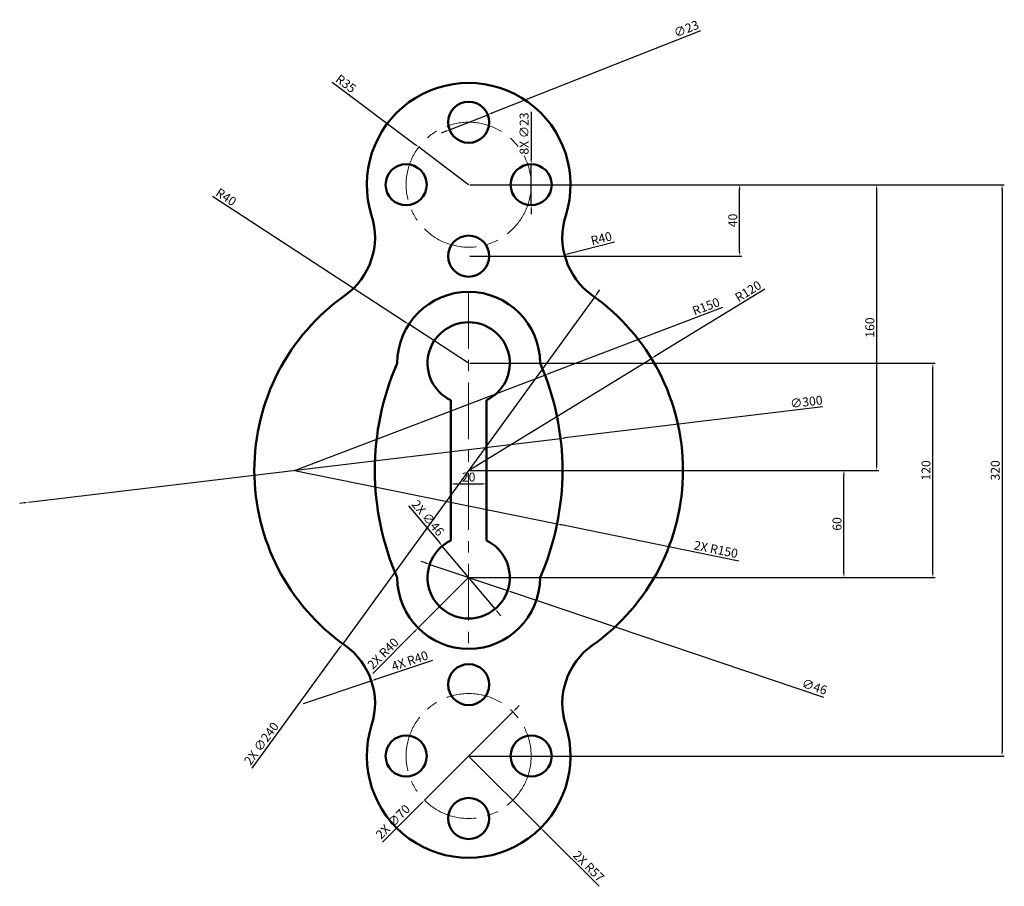
# Model space of a CAD drawing. Units: millimetres. Extents: x 3115 to 3666, y 1639 to 2124.
import ezdxf

# ---------------------------------------------------------------- set-up
doc = ezdxf.new("R2010")
doc.units = ezdxf.units.MM
doc.linetypes.add('CENTER', pattern=[50.8, 31.75, -6.35, 6.35, -6.35])
for name, color, linetype, lineweight in [('M-CNTR', 4, 'CENTER', 18), ('M-DIMS', 2, 'Continuous', 25), ('M-OUTL', 7, 'Continuous', 50)]:
    doc.layers.add(name, color=color, linetype=linetype, lineweight=lineweight)
doc.styles.get("Standard").update_dxf_attribs({"font": 'arial.ttf'})
doc.dimstyles.new('ISO-25', dxfattribs={"dimtxt": 5, "dimasz": 2.5, "dimexe": 1.25, "dimexo": 0.625, "dimtad": 1, "dimtxsty": 'Standard', "dimcen": 2.5, "dimadec": 0, "dimazin": 0, "dimtfac": 1, "dimtmove": 0, "dimatfit": 3, "dimfxl": 1, "dimarcsym": 0})

# ---------------------------------------------------------------- blocks, each defined once
blk = doc.blocks.new('*D1')
at = {"layer": 'Defpoints', "color": 0, "transparency": 16777216}
for p in [(3366.01, 1931.75), (3625.89, 1931.75), (3366.01, 1811.75)]:
    blk.add_point(p, dxfattribs=at)
at = {"layer": 'M-DIMS', "color": 0, "lineweight": -2, "transparency": 16777216}
for p, q in [((3366.63, 1931.75), (3627.14, 1931.75)), ((3625.89, 1814.25), (3625.89, 1929.25)), ((3366.63, 1811.75), (3627.14, 1811.75))]:
    blk.add_line(p, q, dxfattribs=at)
at = {"layer": 'M-DIMS', "color": 0, "transparency": 16777216}
for points in [[(3625.47, 1929.25), (3626.3, 1929.25), (3625.89, 1931.75)], [(3625.47, 1814.25), (3626.3, 1814.25), (3625.89, 1811.75)]]:
    blk.add_solid(points, dxfattribs=at)
at = {"layer": 'M-DIMS', "color": 0, "transparency": 16777216, "insert": (3622.71, 1871.75), "char_height": 5, "attachment_point": 5, "rotation": 90}
blk.add_mtext('120', dxfattribs=at)
blk = doc.blocks.new('*D2')
at = {"layer": 'Defpoints', "color": 0, "transparency": 16777216}
for p in [(3366.01, 1871.75), (3576.08, 1871.75), (3366.01, 1811.75)]:
    blk.add_point(p, dxfattribs=at)
at = {"layer": 'M-DIMS', "color": 0, "lineweight": -2, "transparency": 16777216}
for p, q in [((3366.63, 1871.75), (3577.33, 1871.75)), ((3576.08, 1814.25), (3576.08, 1869.25)), ((3366.63, 1811.75), (3577.33, 1811.75))]:
    blk.add_line(p, q, dxfattribs=at)
at = {"layer": 'M-DIMS', "color": 0, "transparency": 16777216}
for points in [[(3575.66, 1869.25), (3576.5, 1869.25), (3576.08, 1871.75)], [(3575.66, 1814.25), (3576.5, 1814.25), (3576.08, 1811.75)]]:
    blk.add_solid(points, dxfattribs=at)
at = {"layer": 'M-DIMS', "color": 0, "transparency": 16777216, "insert": (3572.9, 1841.75), "char_height": 5, "attachment_point": 5, "rotation": 90}
blk.add_mtext('60', dxfattribs=at)
blk = doc.blocks.new('*D3')
at = {"layer": 'Defpoints', "color": 0, "transparency": 16777216}
for p in [(3366.01, 2031.75), (3594.46, 2031.75), (3366.01, 1871.75)]:
    blk.add_point(p, dxfattribs=at)
at = {"layer": 'M-DIMS', "color": 0, "lineweight": -2, "transparency": 16777216}
for p, q in [((3366.63, 2031.75), (3595.71, 2031.75)), ((3594.46, 1874.25), (3594.46, 2029.25)), ((3366.63, 1871.75), (3595.71, 1871.75))]:
    blk.add_line(p, q, dxfattribs=at)
at = {"layer": 'M-DIMS', "color": 0, "transparency": 16777216}
for points in [[(3594.04, 2029.25), (3594.88, 2029.25), (3594.46, 2031.75)], [(3594.04, 1874.25), (3594.88, 1874.25), (3594.46, 1871.75)]]:
    blk.add_solid(points, dxfattribs=at)
at = {"layer": 'M-DIMS', "color": 0, "transparency": 16777216, "insert": (3591.28, 1951.75), "char_height": 5, "attachment_point": 5, "rotation": 90}
blk.add_mtext('160', dxfattribs=at)
blk = doc.blocks.new('*D4')
at = {"layer": 'Defpoints', "color": 0, "transparency": 16777216}
for p in [(3344.22, 1819.1), (3387.8, 1804.39)]:
    blk.add_point(p, dxfattribs=at)
at = {"layer": 'M-DIMS', "color": 0, "lineweight": -2, "transparency": 16777216}
for p, q in [((3341.85, 1819.9), (3339.48, 1820.7)), ((3344.22, 1819.1), (3387.8, 1804.39)), ((3564.95, 1744.61), (3390.17, 1803.59))]:
    blk.add_line(p, q, dxfattribs=at)
at = {"layer": 'M-DIMS', "color": 0, "transparency": 16777216}
for points in [[(3341.98, 1820.3), (3341.71, 1819.51), (3344.22, 1819.1)], [(3390.3, 1803.99), (3390.04, 1803.2), (3387.8, 1804.39)]]:
    blk.add_solid(points, dxfattribs=at)
at = {"layer": 'M-DIMS', "color": 0, "transparency": 16777216, "insert": (3559.45, 1749.97), "char_height": 5, "attachment_point": 5, "rotation": 341.3529}
blk.add_mtext('∅46', dxfattribs=at)
blk = doc.blocks.new('*D5')
at = {"layer": 'Defpoints', "color": 0, "transparency": 16777216}
for p in [(3417.46, 1889.63), (3119.6, 1853.86)]:
    blk.add_point(p, dxfattribs=at)
at = {"layer": 'M-DIMS', "color": 0, "lineweight": -2, "transparency": 16777216}
for p, q in [((3564.34, 1907.27), (3419.94, 1889.93)), ((3119.6, 1853.86), (3417.46, 1889.63)), ((3117.12, 1853.56), (3114.64, 1853.26))]:
    blk.add_line(p, q, dxfattribs=at)
at = {"layer": 'M-DIMS', "color": 0, "transparency": 16777216}
for points in [[(3419.89, 1890.35), (3419.99, 1889.52), (3417.46, 1889.63)], [(3117.07, 1853.98), (3117.17, 1853.15), (3119.6, 1853.86)]]:
    blk.add_solid(points, dxfattribs=at)
at = {"layer": 'M-DIMS', "color": 0, "transparency": 16777216, "insert": (3555.15, 1909.51), "char_height": 5, "attachment_point": 5, "rotation": 6.8485}
blk.add_mtext('∅300', dxfattribs=at)
blk = doc.blocks.new('*D6')
at = {"layer": 'Defpoints', "color": 0, "transparency": 16777216}
for p in [(3376.71, 2070.97), (3355.31, 2062.53)]:
    blk.add_point(p, dxfattribs=at)
at = {"layer": 'M-DIMS', "color": 0, "lineweight": -2, "transparency": 16777216}
for p, q in [((3495.76, 2117.96), (3379.03, 2071.89)), ((3355.31, 2062.53), (3376.71, 2070.97)), ((3352.99, 2061.61), (3350.66, 2060.69))]:
    blk.add_line(p, q, dxfattribs=at)
at = {"layer": 'M-DIMS', "color": 0, "transparency": 16777216}
for points in [[(3378.88, 2072.28), (3379.18, 2071.5), (3376.71, 2070.97)], [(3352.83, 2061.99), (3353.14, 2061.22), (3355.31, 2062.53)]]:
    blk.add_solid(points, dxfattribs=at)
at = {"layer": 'M-DIMS', "color": 0, "transparency": 16777216, "insert": (3488.09, 2118.5), "char_height": 5, "attachment_point": 5, "rotation": 21.5398}
blk.add_mtext('∅23', dxfattribs=at)
blk = doc.blocks.new('*D7')
at = {"layer": 'Defpoints', "color": 0, "transparency": 16777216}
for p in [(3458.45, 2002.34), (3419.67, 1992.52)]:
    blk.add_point(p, dxfattribs=at)
at = {"layer": 'M-DIMS', "color": 0, "lineweight": -2, "transparency": 16777216}
blk.add_line((3447.6, 1999.59), (3422.09, 1993.13), dxfattribs=at)
at = {"layer": 'M-DIMS', "color": 0, "transparency": 16777216}
blk.add_solid([(3421.99, 1993.53), (3422.2, 1992.73), (3419.67, 1992.52)], dxfattribs=at)
at = {"layer": 'M-DIMS', "color": 0, "transparency": 16777216, "insert": (3440.43, 2001.06), "char_height": 5, "attachment_point": 5, "rotation": 14.2239}
blk.add_mtext('R40', dxfattribs=at)
blk = doc.blocks.new('*D8')
at = {"layer": 'Defpoints', "color": 0, "transparency": 16777216}
for p in [(3468.33, 1934.44), (3366.01, 1871.75)]:
    blk.add_point(p, dxfattribs=at)
at = {"layer": 'M-DIMS', "color": 0, "lineweight": -2, "transparency": 16777216}
for p, q in [((3531.75, 1973.29), (3470.46, 1935.74)), ((3366.01, 1871.75), (3468.33, 1934.44))]:
    blk.add_line(p, q, dxfattribs=at)
at = {"layer": 'M-DIMS', "color": 0, "transparency": 16777216}
blk.add_solid([(3470.25, 1936.1), (3470.68, 1935.39), (3468.33, 1934.44)], dxfattribs=at)
at = {"layer": 'M-DIMS', "color": 0, "transparency": 16777216, "insert": (3522.82, 1971.55), "char_height": 5, "attachment_point": 5, "rotation": 31.4946}
blk.add_mtext('R120', dxfattribs=at)
blk = doc.blocks.new('*D9')
at = {"layer": 'Defpoints', "color": 0, "transparency": 16777216}
for p in [(3408.71, 1925.14), (3268.53, 1871.75)]:
    blk.add_point(p, dxfattribs=at)
at = {"layer": 'M-DIMS', "color": 0, "lineweight": -2, "transparency": 16777216}
for p, q in [((3508.21, 1963.04), (3411.04, 1926.03)), ((3268.53, 1871.75), (3408.71, 1925.14))]:
    blk.add_line(p, q, dxfattribs=at)
at = {"layer": 'M-DIMS', "color": 0, "transparency": 16777216}
blk.add_solid([(3410.9, 1926.42), (3411.19, 1925.64), (3408.71, 1925.14)], dxfattribs=at)
at = {"layer": 'M-DIMS', "color": 0, "transparency": 16777216, "insert": (3499.11, 1962.97), "char_height": 5, "attachment_point": 5, "rotation": 20.8517}
blk.add_mtext('R150', dxfattribs=at)
blk = doc.blocks.new('*D10')
at = {"layer": 'Defpoints', "color": 0, "transparency": 16777216}
for p in [(3338.06, 2052.81), (3366.01, 2031.75)]:
    blk.add_point(p, dxfattribs=at)
at = {"layer": 'M-DIMS', "color": 0, "lineweight": -2, "transparency": 16777216}
for p, q in [((3289.66, 2089.29), (3336.06, 2054.32)), ((3366.01, 2031.75), (3338.06, 2052.81))]:
    blk.add_line(p, q, dxfattribs=at)
at = {"layer": 'M-DIMS', "color": 0, "transparency": 16777216}
blk.add_solid([(3336.31, 2054.65), (3335.81, 2053.99), (3338.06, 2052.81)], dxfattribs=at)
at = {"layer": 'M-DIMS', "color": 0, "transparency": 16777216, "insert": (3296.86, 2087.85), "char_height": 5, "attachment_point": 5, "rotation": 322.9931}
blk.add_mtext('R35', dxfattribs=at)
blk = doc.blocks.new('*D11')
at = {"layer": 'Defpoints', "color": 0, "transparency": 16777216}
for p in [(3332.51, 1953.6), (3366.01, 1931.75)]:
    blk.add_point(p, dxfattribs=at)
at = {"layer": 'M-DIMS', "color": 0, "lineweight": -2, "transparency": 16777216}
for p, q in [((3222.62, 2025.28), (3330.41, 1954.97)), ((3366.01, 1931.75), (3332.51, 1953.6))]:
    blk.add_line(p, q, dxfattribs=at)
at = {"layer": 'M-DIMS', "color": 0, "transparency": 16777216}
blk.add_solid([(3330.64, 1955.32), (3330.18, 1954.62), (3332.51, 1953.6)], dxfattribs=at)
at = {"layer": 'M-DIMS', "color": 0, "transparency": 16777216, "insert": (3229.87, 2024.34), "char_height": 5, "attachment_point": 5, "rotation": 326.8847}
blk.add_mtext('R40', dxfattribs=at)
blk = doc.blocks.new('*D12')
at = {"layer": 'Defpoints', "color": 0, "transparency": 16777216}
for p in [(3366.01, 2031.75), (3366.01, 1711.75), (3664.66, 1711.75)]:
    blk.add_point(p, dxfattribs=at)
at = {"layer": 'M-DIMS', "color": 0, "lineweight": -2, "transparency": 16777216}
for p, q in [((3366.63, 2031.75), (3665.91, 2031.75)), ((3664.66, 2029.25), (3664.66, 1714.25)), ((3366.63, 1711.75), (3665.91, 1711.75))]:
    blk.add_line(p, q, dxfattribs=at)
at = {"layer": 'M-DIMS', "color": 0, "transparency": 16777216}
for points in [[(3664.24, 2029.25), (3665.07, 2029.25), (3664.66, 2031.75)], [(3664.24, 1714.25), (3665.07, 1714.25), (3664.66, 1711.75)]]:
    blk.add_solid(points, dxfattribs=at)
at = {"layer": 'M-DIMS', "color": 0, "transparency": 16777216, "insert": (3661.48, 1871.75), "char_height": 5, "attachment_point": 5, "rotation": 90}
blk.add_mtext('320', dxfattribs=at)
blk = doc.blocks.new('FLANGE-HOLE-PATTERN-4X23')
for centre in [(0, 35), (-35, 0), (35, 0), (0, -40)]:
    blk.add_circle(centre, 11.5)
blk = doc.blocks.new('*D14')
at = {"layer": 'Defpoints', "color": 0, "transparency": 16777216}
for p in [(3376.01, 1864.16), (3356.01, 1832.46), (3376.01, 1832.46)]:
    blk.add_point(p, dxfattribs=at)
at = {"layer": 'M-DIMS', "color": 0, "lineweight": -2, "transparency": 16777216}
for p, q in [((3356.01, 1833.08), (3356.01, 1865.41)), ((3358.51, 1864.16), (3373.51, 1864.16)), ((3376.01, 1833.08), (3376.01, 1865.41))]:
    blk.add_line(p, q, dxfattribs=at)
at = {"layer": 'M-DIMS', "color": 0, "transparency": 16777216}
for points in [[(3358.51, 1864.58), (3358.51, 1863.74), (3356.01, 1864.16)], [(3373.51, 1864.58), (3373.51, 1863.74), (3376.01, 1864.16)]]:
    blk.add_solid(points, dxfattribs=at)
at = {"layer": 'M-DIMS', "color": 0, "transparency": 16777216, "insert": (3366.01, 1867.34), "char_height": 5, "attachment_point": 5}
blk.add_mtext('20', dxfattribs=at)
blk = doc.blocks.new('*D15')
at = {"layer": 'Defpoints', "color": 0, "transparency": 16777216}
for p in [(3366.01, 2031.75), (3517.71, 2031.75), (3366.01, 1991.75)]:
    blk.add_point(p, dxfattribs=at)
at = {"layer": 'M-DIMS', "color": 0, "lineweight": -2, "transparency": 16777216}
for p, q in [((3366.63, 2031.75), (3518.96, 2031.75)), ((3517.71, 1994.25), (3517.71, 2029.25)), ((3366.63, 1991.75), (3518.96, 1991.75))]:
    blk.add_line(p, q, dxfattribs=at)
at = {"layer": 'M-DIMS', "color": 0, "transparency": 16777216}
for points in [[(3517.29, 2029.25), (3518.13, 2029.25), (3517.71, 2031.75)], [(3517.29, 1994.25), (3518.13, 1994.25), (3517.71, 1991.75)]]:
    blk.add_solid(points, dxfattribs=at)
at = {"layer": 'M-DIMS', "color": 0, "transparency": 16777216, "insert": (3514.53, 2011.75), "char_height": 5, "attachment_point": 5, "rotation": 90}
blk.add_mtext('40', dxfattribs=at)
blk = doc.blocks.new('*D16')
at = {"layer": 'Defpoints', "color": 0, "transparency": 16777216}
for p in [(3436.54, 1968.83), (3295.48, 1774.67)]:
    blk.add_point(p, dxfattribs=at)
at = {"layer": 'M-DIMS', "color": 0, "lineweight": -2, "transparency": 16777216}
for p, q in [((3436.54, 1968.83), (3295.48, 1774.67)), ((3438.01, 1970.85), (3439.48, 1972.87)), ((3244.84, 1704.98), (3294.01, 1772.64))]:
    blk.add_line(p, q, dxfattribs=at)
at = {"layer": 'M-DIMS', "color": 0, "transparency": 16777216}
for points in [[(3437.68, 1971.1), (3438.35, 1970.61), (3436.54, 1968.83)], [(3293.67, 1772.89), (3294.34, 1772.4), (3295.48, 1774.67)]]:
    blk.add_solid(points, dxfattribs=at)
at = {"layer": 'M-DIMS', "color": 0, "transparency": 16777216, "insert": (3250.47, 1718.37), "char_height": 5, "attachment_point": 5, "rotation": 54.0002}
blk.add_mtext('2X ∅240', dxfattribs=at)
blk = doc.blocks.new('*D17')
at = {"layer": 'Defpoints', "color": 0, "transparency": 16777216}
for p in [(3366.01, 1711.75), (3406.31, 1671.44)]:
    blk.add_point(p, dxfattribs=at)
at = {"layer": 'M-DIMS', "color": 0, "lineweight": -2, "transparency": 16777216}
for p, q in [((3366.01, 1711.75), (3406.31, 1671.44)), ((3438.99, 1638.76), (3408.08, 1669.67))]:
    blk.add_line(p, q, dxfattribs=at)
at = {"layer": 'M-DIMS', "color": 0, "transparency": 16777216}
blk.add_solid([(3408.38, 1669.97), (3407.79, 1669.38), (3406.31, 1671.44)], dxfattribs=at)
at = {"layer": 'M-DIMS', "color": 0, "transparency": 16777216, "insert": (3432.74, 1649.51), "char_height": 5, "attachment_point": 5, "rotation": 314.9997}
blk.add_mtext('2X R57', dxfattribs=at)
blk = doc.blocks.new('*D18')
at = {"layer": 'Defpoints', "color": 0, "transparency": 16777216}
for p in [(3311.5, 1753.86), (3273.57, 1741.15)]:
    blk.add_point(p, dxfattribs=at)
at = {"layer": 'M-DIMS', "color": 0, "lineweight": -2, "transparency": 16777216}
for p, q in [((3345.69, 1765.32), (3313.87, 1754.66)), ((3273.57, 1741.15), (3311.5, 1753.86))]:
    blk.add_line(p, q, dxfattribs=at)
at = {"layer": 'M-DIMS', "color": 0, "transparency": 16777216}
blk.add_solid([(3313.74, 1755.05), (3314, 1754.26), (3311.5, 1753.86)], dxfattribs=at)
at = {"layer": 'M-DIMS', "color": 0, "transparency": 16777216, "insert": (3333.24, 1764.5), "char_height": 5, "attachment_point": 5, "rotation": 18.5305}
blk.add_mtext('4X R40', dxfattribs=at)
blk = doc.blocks.new('*D19')
at = {"layer": 'Defpoints', "color": 0, "transparency": 16777216}
for p in [(3268.53, 1871.75), (3415.5, 1841.75)]:
    blk.add_point(p, dxfattribs=at)
at = {"layer": 'M-DIMS', "color": 0, "lineweight": -2, "transparency": 16777216}
for p, q in [((3268.53, 1871.75), (3415.5, 1841.75)), ((3517.35, 1820.95), (3417.95, 1841.25))]:
    blk.add_line(p, q, dxfattribs=at)
at = {"layer": 'M-DIMS', "color": 0, "transparency": 16777216}
blk.add_solid([(3418.03, 1841.65), (3417.87, 1840.84), (3415.5, 1841.75)], dxfattribs=at)
at = {"layer": 'M-DIMS', "color": 0, "transparency": 16777216, "insert": (3504.32, 1826.86), "char_height": 5, "attachment_point": 5, "rotation": 348.4622}
blk.add_mtext('2X R150', dxfattribs=at)
blk = doc.blocks.new('*D20')
at = {"layer": 'Defpoints', "color": 0, "transparency": 16777216}
for p in [(3366.01, 1811.75), (3337.72, 1783.46)]:
    blk.add_point(p, dxfattribs=at)
at = {"layer": 'M-DIMS', "color": 0, "lineweight": -2, "transparency": 16777216}
for p, q in [((3366.01, 1811.75), (3337.72, 1783.46)), ((3312.27, 1758), (3335.96, 1781.7))]:
    blk.add_line(p, q, dxfattribs=at)
at = {"layer": 'M-DIMS', "color": 0, "transparency": 16777216}
blk.add_solid([(3335.66, 1781.99), (3336.25, 1781.4), (3337.72, 1783.46)], dxfattribs=at)
at = {"layer": 'M-DIMS', "color": 0, "transparency": 16777216, "insert": (3318.51, 1768.74), "char_height": 5, "attachment_point": 5, "rotation": 45.0005}
blk.add_mtext('2X R40', dxfattribs=at)
blk = doc.blocks.new('*D21')
at = {"layer": 'Defpoints', "color": 0, "transparency": 16777216}
for p in [(3351.22, 1829.37), (3380.79, 1794.13)]:
    blk.add_point(p, dxfattribs=at)
at = {"layer": 'M-DIMS', "color": 0, "lineweight": -2, "transparency": 16777216}
for p, q in [((3332.32, 1851.9), (3349.62, 1831.28)), ((3380.79, 1794.13), (3351.22, 1829.37)), ((3382.4, 1792.21), (3384.01, 1790.3))]:
    blk.add_line(p, q, dxfattribs=at)
at = {"layer": 'M-DIMS', "color": 0, "transparency": 16777216}
for points in [[(3349.94, 1831.55), (3349.3, 1831.01), (3351.22, 1829.37)], [(3382.72, 1792.48), (3382.08, 1791.95), (3380.79, 1794.13)]]:
    blk.add_solid(points, dxfattribs=at)
at = {"layer": 'M-DIMS', "color": 0, "transparency": 16777216, "insert": (3342.71, 1844.68), "char_height": 5, "attachment_point": 5, "rotation": 310.0022}
blk.add_mtext('2X ∅46', dxfattribs=at)
blk = doc.blocks.new('*D22')
at = {"layer": 'Defpoints', "color": 0, "transparency": 16777216}
for p in [(3390.76, 1736.5), (3341.26, 1687)]:
    blk.add_point(p, dxfattribs=at)
at = {"layer": 'M-DIMS', "color": 0, "lineweight": -2, "transparency": 16777216}
for p, q in [((3392.53, 1738.26), (3394.29, 1740.03)), ((3390.76, 1736.5), (3341.26, 1687)), ((3317.79, 1663.52), (3339.49, 1685.23))]:
    blk.add_line(p, q, dxfattribs=at)
at = {"layer": 'M-DIMS', "color": 0, "transparency": 16777216}
for points in [[(3392.23, 1738.56), (3392.82, 1737.97), (3390.76, 1736.5)], [(3339.2, 1685.53), (3339.79, 1684.94), (3341.26, 1687)]]:
    blk.add_solid(points, dxfattribs=at)
at = {"layer": 'M-DIMS', "color": 0, "transparency": 16777216, "insert": (3324.07, 1674.5), "char_height": 5, "attachment_point": 5, "rotation": 45.0006}
blk.add_mtext('2X ∅70', dxfattribs=at)
blk = doc.blocks.new('*D23')
at = {"layer": 'Defpoints', "color": 0, "transparency": 16777216}
for p in [(3401.01, 2043.25), (3401.01, 2020.25)]:
    blk.add_point(p, dxfattribs=at)
at = {"layer": 'M-DIMS', "color": 0, "lineweight": -2, "transparency": 16777216}
for p, q in [((3401.01, 2072.58), (3401.01, 2045.75)), ((3401.01, 2020.25), (3401.01, 2043.25)), ((3401.01, 2017.75), (3401.01, 2015.25))]:
    blk.add_line(p, q, dxfattribs=at)
at = {"layer": 'M-DIMS', "color": 0, "transparency": 16777216}
for points in [[(3400.59, 2045.75), (3401.43, 2045.75), (3401.01, 2043.25)], [(3400.59, 2017.75), (3401.43, 2017.75), (3401.01, 2020.25)]]:
    blk.add_solid(points, dxfattribs=at)
at = {"layer": 'M-DIMS', "color": 0, "transparency": 16777216, "insert": (3397.69, 2060.42), "char_height": 5, "attachment_point": 5, "rotation": 90}
blk.add_mtext('8X ∅23', dxfattribs=at)

msp = doc.modelspace()

# ---------------------------------------------------------------- linework, layer by layer
at = {"layer": 'M-CNTR'}
msp.add_line((3366.009, 1971.747), (3366.009, 1771.747), dxfattribs=at)
for centre in [(3366.009, 2031.747), (3366.009, 1711.747)]:
    msp.add_circle(centre, 35, dxfattribs=at)
at = {"layer": 'M-OUTL'}
for p, q in [((3356.009, 1832.46), (3356.009, 1911.035)), ((3376.009, 1832.46), (3376.009, 1911.035))]:
    msp.add_line(p, q, dxfattribs=at)
for centre, radius, start, end in [((3366.009, 2031.747), 57, 342.35461, 197.64539), ((3273.573, 2002.344), 40, 305.29079, 17.64539), ((3458.445, 2002.344), 40, 162.35461, 234.70921), ((3366.009, 1871.747), 120, 125.29079, 234.70921), ((3366.009, 1931.747), 40, 0, 180), ((3366.009, 1871.747), 120, 305.29079, 54.70921), ((3366.009, 1931.747), 23, 295.77146, 244.22854), ((3463.486, 1871.747), 150, 156.42182, 203.57818), ((3268.532, 1871.747), 150, 336.42182, 23.57818), ((3366.009, 1811.747), 23, 115.77146, 64.22854), ((3366.009, 1811.747), 40, 180, 0), ((3273.573, 1741.151), 40, 342.35461, 54.70921), ((3458.445, 1741.151), 40, 125.29079, 197.64539), ((3366.009, 1711.747), 57, 162.35461, 17.64539)]:
    msp.add_arc(centre, radius, start, end, dxfattribs=at)

# ---------------------------------------------------------------- block references
msp.add_blockref('FLANGE-HOLE-PATTERN-4X23', (3366.009, 2031.747), dxfattribs=at)
at = {"layer": 'M-OUTL', "rotation": 180}
msp.add_blockref('FLANGE-HOLE-PATTERN-4X23', (3366.009, 1711.747), dxfattribs=at)

# ---------------------------------------------------------------- dimensions: what is measured, and where the dimension line sits
at = {"layer": 'M-DIMS'}
for p1, p2, picture, middle in [((3355.312, 2062.525), (3376.706, 2070.97), '*D6', (3489.313, 2115.417)), ((3119.602, 1853.861), (3417.461, 1889.634), '*D5', (3555.542, 1906.218)), ((3344.216, 1819.101), (3387.802, 1804.394), '*D4', (3558.39, 1746.828))]:
    dim = msp.add_diameter_dim_2p(p1=p1, p2=p2, dimstyle='ISO-25', override={"dimclrd": 0, "dimclre": 0, "dimclrt": 0}, dxfattribs=at)
    dim.commit()
    dim.dimension.update_dxf_attribs({"geometry": picture, "text_midpoint": middle, "dimtype": 163})
for center, mpoint, picture, middle in [((3366.009, 2031.747), (3338.059, 2052.814), '*D10', (3294.948, 2085.309)), ((3366.009, 1931.747), (3332.506, 1953.601), '*D11', (3228.137, 2021.677)), ((3458.445, 2002.344), (3419.672, 1992.516), '*D7', (3441.209, 1997.975)), ((3366.009, 1871.747), (3468.332, 1934.438), '*D8', (3524.479, 1968.837)), ((3268.532, 1871.747), (3408.707, 1925.14), '*D9', (3500.237, 1960.003))]:
    dim = msp.add_radius_dim(center=center, mpoint=mpoint, dimstyle='ISO-25', override={"dimclrd": 0, "dimclre": 0, "dimclrt": 0}, dxfattribs=at)
    dim.commit()
    dim.dimension.update_dxf_attribs({"geometry": picture, "text_midpoint": middle, "dimtype": 164})
dim = msp.add_diameter_dim_2p(p1=(3401.009, 2020.247), p2=(3401.009, 2043.247), text='8X <>', dimstyle='ISO-25', override={"dimdec": 0, "dimlfac": 1, "dimrnd": 0, "dimzin": 0, "dimdsep": 46, "dimlunit": 2}, dxfattribs=at)
dim.commit()
dim.dimension.update_dxf_attribs({"geometry": '*D23', "text_midpoint": (3401.009, 2060.416)})
for base, p1, p2, override, picture, middle in [((3594.46, 2031.747), (3366.009, 1871.747), (3366.009, 2031.747), {"dimclrd": 0, "dimclre": 0, "dimclrt": 0}, '*D3', (3591.282, 1951.747)), ((3664.658, 1711.747), (3366.009, 2031.747), (3366.009, 1711.747), {"dimclrd": 0, "dimclre": 0, "dimclrt": 0}, '*D12', (3661.478, 1871.747)), ((3517.709, 2031.747), (3366.009, 1991.747), (3366.009, 2031.747), {"dimdec": 0, "dimlfac": 1, "dimrnd": 0, "dimzin": 0, "dimdsep": 46, "dimlunit": 2}, '*D15', (3514.531, 2011.747)), ((3625.885, 1931.747), (3366.009, 1811.747), (3366.009, 1931.747), {"dimclrd": 0, "dimclre": 0, "dimclrt": 0}, '*D1', (3622.707, 1871.747)), ((3576.081, 1871.747), (3366.009, 1811.747), (3366.009, 1871.747), {"dimclrd": 0, "dimclre": 0, "dimclrt": 0}, '*D2', (3572.903, 1841.747))]:
    dim = msp.add_linear_dim(base=base, p1=p1, p2=p2, angle=90, dimstyle='ISO-25', override=override, dxfattribs=at)
    dim.commit()
    dim.dimension.update_dxf_attribs({"geometry": picture, "text_midpoint": middle})
for p1, p2, picture, middle in [((3436.543, 1968.83), (3295.475, 1774.665), '*D16', (3253.155, 1716.416)), ((3380.794, 1794.129), (3351.224, 1829.366), '*D21', (3340.164, 1842.546)), ((3390.757, 1736.496), (3341.261, 1686.999), '*D22', (3326.411, 1672.149))]:
    dim = msp.add_diameter_dim_2p(p1=p1, p2=p2, text='2X <>', dimstyle='ISO-25', override={"dimdec": 0, "dimlfac": 1, "dimrnd": 0, "dimzin": 0, "dimdsep": 46, "dimlunit": 2}, dxfattribs=at)
    dim.commit()
    dim.dimension.update_dxf_attribs({"geometry": picture, "text_midpoint": middle, "dimtype": 163})
for center, mpoint, text, picture, middle in [((3268.532, 1871.747), (3415.501, 1841.745), '2X <>', '*D19', (3503.682, 1823.744)), ((3366.009, 1811.747), (3337.725, 1783.463), '2X <>', '*D20', (3320.755, 1766.492)), ((3273.573, 1741.151), (3311.499, 1753.863), '4X <>', '*D18', (3334.255, 1761.49)), ((3366.009, 1711.747), (3406.314, 1671.442), '2X <>', '*D17', (3430.497, 1647.259))]:
    dim = msp.add_radius_dim(center=center, mpoint=mpoint, text=text, dimstyle='ISO-25', override={"dimdec": 0, "dimlfac": 1, "dimrnd": 0, "dimzin": 0, "dimdsep": 46, "dimlunit": 2}, dxfattribs=at)
    dim.commit()
    dim.dimension.update_dxf_attribs({"geometry": picture, "text_midpoint": middle, "dimtype": 164})
dim = msp.add_linear_dim(base=(3376.009, 1864.16), p1=(3356.009, 1832.46), p2=(3376.009, 1832.46), dimstyle='ISO-25', override={"dimdec": 0, "dimlfac": 1, "dimrnd": 0, "dimzin": 0, "dimdsep": 46, "dimlunit": 2}, dxfattribs=at)
dim.commit()
dim.dimension.update_dxf_attribs({"geometry": '*D14', "text_midpoint": (3366.009, 1867.338)})

doc.saveas('drawing.dxf')
